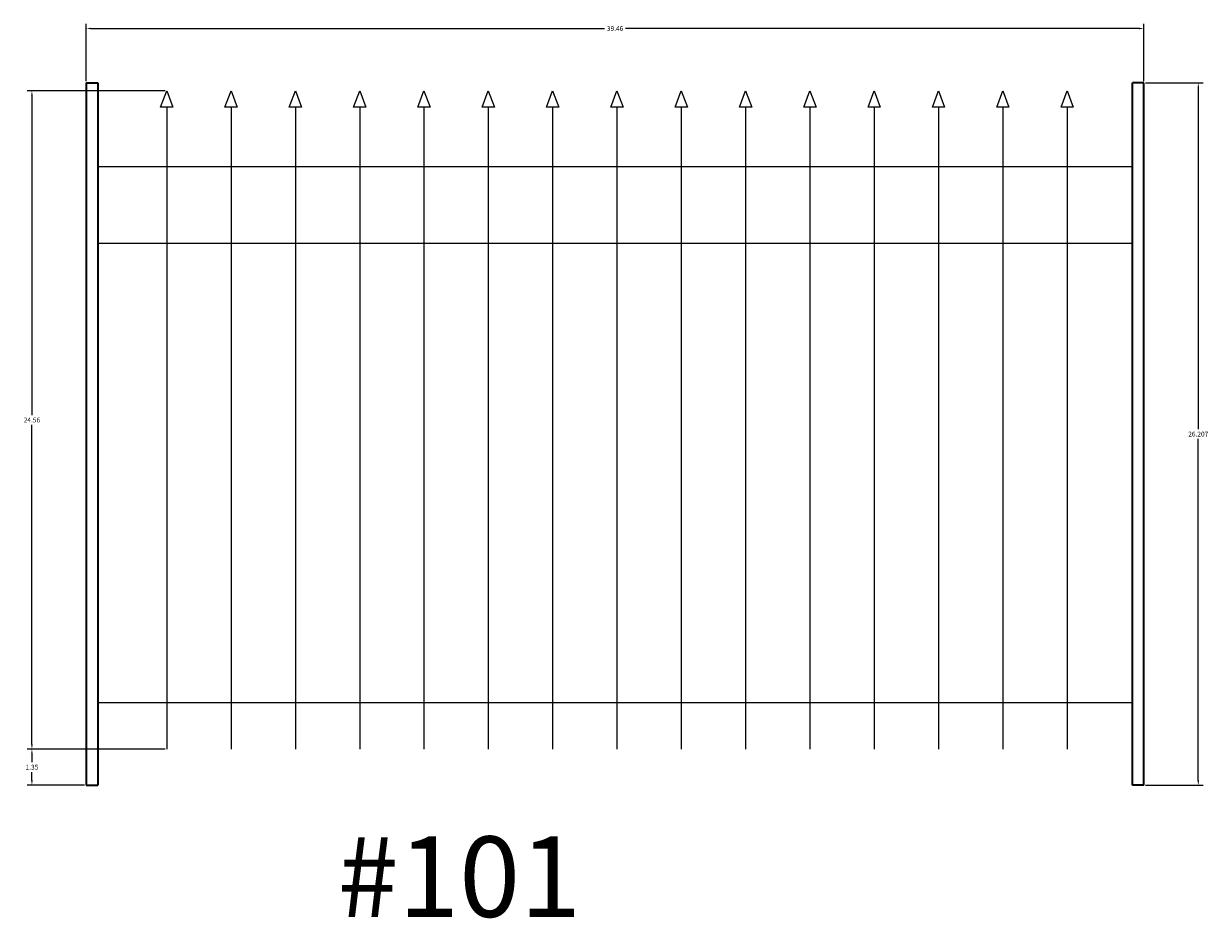
# Model space of a CAD drawing. Units: inches. Extents: x 756 to 915, y 488 to 695.
# Tile 20 of 25: x 815 to 859, y 661 to 694. Entities that reach past the tile are written whole.
import ezdxf

# ---------------------------------------------------------------- set-up
doc = ezdxf.new("R2010")
doc.units = ezdxf.units.IN
doc.header["$MEASUREMENT"] = 0
for name, color, linetype, lineweight in [('L-ANNO-TEXT', 7, 'Continuous', 25), ('L-FENC-PCKT', 7, 'Continuous', 18), ('L-FENC-POST', 7, 'Continuous', 35), ('L-FENC-RAIL', 7, 'Continuous', 25), ('M-DIMS', 2, 'Continuous', 18)]:
    doc.layers.add(name, color=color, linetype=linetype, lineweight=lineweight)
doc.styles.get("Standard").update_dxf_attribs({"font": 'arial.ttf'})
doc.dimstyles.get("Standard").update_dxf_attribs({"dimtxt": 0.18, "dimasz": 0.18, "dimexe": 0.18, "dimexo": 0.0625, "dimgap": 0.09, "dimtad": 0, "dimtih": 1, "dimtoh": 1, "dimdec": 0, "dimzin": 0, "dimdsep": 46, "dimlunit": 3, "dimtxsty": 'Standard', "dimcen": 0.09, "dimadec": 0, "dimazin": 0, "dimtfac": 1, "dimtdec": 0, "dimtofl": 0, "dimtmove": 0, "dimatfit": 3, "dimfxl": 1, "dimtolj": 1, "dimtzin": 0, "dimarcsym": 0})

# ---------------------------------------------------------------- blocks, each defined once
blk = doc.blocks.new('PICKET-SPEAR-EXTENDED')
blk.add_line((0.228, 23.946), (0.228, 0))
blk.add_lwpolyline([(0.228, 23.946), (0, 23.946), (0.228, 24.558), (0.455, 23.946)], close=True)
blk = doc.blocks.new('FENCE-POST-LEFT')
for p, q in [((0, 26.207), (0, 0)), ((0, 26.207), (0.426, 26.207)), ((0.426, 26.207), (0.426, 0)), ((0.426, 26.207), (0.426, 0)), ((0, 0), (0.426, 0))]:
    blk.add_line(p, q)
blk = doc.blocks.new('FENCE-POST-RIGHT')
for p, q in [((0, 26.207), (0, 0)), ((0, 26.207), (0.427, 26.207)), ((0.427, 26.207), (0.427, 0)), ((0, 0), (0.427, 0))]:
    blk.add_line(p, q)
blk = doc.blocks.new('*D19')
at = {"layer": 'Defpoints', "color": 0, "transparency": 16777216}
for p in [(856.698, 693.983), (817.24, 691.953), (856.698, 691.953)]:
    blk.add_point(p, dxfattribs=at)
at = {"layer": 'M-DIMS', "color": 0, "lineweight": -2, "transparency": 16777216}
for p, q in [((817.24, 692.015), (817.24, 694.163)), ((817.42, 693.983), (836.575, 693.983)), ((856.518, 693.983), (837.362, 693.983)), ((856.698, 692.015), (856.698, 694.163))]:
    blk.add_line(p, q, dxfattribs=at)
at = {"layer": 'M-DIMS', "color": 0, "transparency": 16777216}
for points in [[(817.42, 694.013), (817.42, 693.953), (817.24, 693.983)], [(856.518, 694.013), (856.518, 693.953), (856.698, 693.983)]]:
    blk.add_solid(points, dxfattribs=at)
at = {"layer": 'M-DIMS', "color": 0, "transparency": 16777216, "insert": (836.969, 693.983), "char_height": 0.18, "attachment_point": 5}
blk.add_mtext('\\A1;39.46', dxfattribs=at)
blk = doc.blocks.new('*D20')
at = {"layer": 'Defpoints', "color": 0, "transparency": 16777216}
for p in [(856.698, 691.953), (858.728, 691.953), (856.698, 665.746)]:
    blk.add_point(p, dxfattribs=at)
at = {"layer": 'M-DIMS', "color": 0, "lineweight": -2, "transparency": 16777216}
for p, q in [((856.76, 691.953), (858.908, 691.953)), ((858.728, 691.773), (858.728, 679.031)), ((858.728, 665.926), (858.728, 678.668)), ((856.76, 665.746), (858.908, 665.746))]:
    blk.add_line(p, q, dxfattribs=at)
at = {"layer": 'M-DIMS', "color": 0, "transparency": 16777216}
for points in [[(858.698, 691.773), (858.758, 691.773), (858.728, 691.953)], [(858.698, 665.926), (858.758, 665.926), (858.728, 665.746)]]:
    blk.add_solid(points, dxfattribs=at)
at = {"layer": 'M-DIMS', "color": 0, "transparency": 16777216, "insert": (858.728, 678.849), "char_height": 0.18, "attachment_point": 5}
blk.add_mtext('\\A1;26.207', dxfattribs=at)
blk = doc.blocks.new('*D21')
at = {"layer": 'Defpoints', "color": 0, "transparency": 16777216}
for p in [(815.21, 691.654), (820.239, 691.654), (820.239, 667.096)]:
    blk.add_point(p, dxfattribs=at)
at = {"layer": 'M-DIMS', "color": 0, "lineweight": -2, "transparency": 16777216}
for p, q in [((820.176, 691.654), (815.03, 691.654)), ((815.21, 691.474), (815.21, 679.557)), ((815.21, 667.276), (815.21, 679.193)), ((820.176, 667.096), (815.03, 667.096))]:
    blk.add_line(p, q, dxfattribs=at)
at = {"layer": 'M-DIMS', "color": 0, "transparency": 16777216}
for points in [[(815.18, 691.474), (815.24, 691.474), (815.21, 691.654)], [(815.18, 667.276), (815.24, 667.276), (815.21, 667.096)]]:
    blk.add_solid(points, dxfattribs=at)
at = {"layer": 'M-DIMS', "color": 0, "transparency": 16777216, "insert": (815.21, 679.375), "char_height": 0.18, "attachment_point": 5}
blk.add_mtext('\\A1;24.56', dxfattribs=at)
blk = doc.blocks.new('*D22')
at = {"layer": 'Defpoints', "color": 0, "transparency": 16777216}
for p in [(815.21, 667.096), (820.239, 667.096), (817.24, 665.746)]:
    blk.add_point(p, dxfattribs=at)
at = {"layer": 'M-DIMS', "color": 0, "lineweight": -2, "transparency": 16777216}
for p, q in [((820.176, 667.096), (815.03, 667.096)), ((815.21, 666.916), (815.21, 666.603)), ((815.21, 665.926), (815.21, 666.239)), ((817.177, 665.746), (815.03, 665.746))]:
    blk.add_line(p, q, dxfattribs=at)
at = {"layer": 'M-DIMS', "color": 0, "transparency": 16777216}
for points in [[(815.18, 666.916), (815.24, 666.916), (815.21, 667.096)], [(815.18, 665.926), (815.24, 665.926), (815.21, 665.746)]]:
    blk.add_solid(points, dxfattribs=at)
at = {"layer": 'M-DIMS', "color": 0, "transparency": 16777216, "insert": (815.21, 666.421), "char_height": 0.18, "attachment_point": 5}
blk.add_mtext('\\A1;1.35', dxfattribs=at)

msp = doc.modelspace()

# ---------------------------------------------------------------- linework, layer by layer
at = {"layer": 'L-FENC-RAIL'}
for p, q in [((817.6662, 688.8379), (856.271, 688.8379)), ((817.6662, 685.9735), (856.271, 685.9735)), ((817.6662, 668.8277), (856.271, 668.8277))]:
    msp.add_line(p, q, dxfattribs=at)

# ---------------------------------------------------------------- block references
at = {"layer": 'L-FENC-PCKT'}
for p in [(820.011, 667.096), (822.4109, 667.096), (824.8108, 667.096), (827.2108, 667.096), (829.6107, 667.096), (832.0106, 667.096), (834.4105, 667.096), (836.8104, 667.096), (839.2103, 667.096), (841.6102, 667.096), (844.0101, 667.096), (846.41, 667.096), (848.81, 667.096), (851.2099, 667.096), (853.6098, 667.096)]:
    msp.add_blockref('PICKET-SPEAR-EXTENDED', p, dxfattribs=at)
at = {"layer": 'L-FENC-POST'}
msp.add_blockref('FENCE-POST-LEFT', (817.2399, 665.746), dxfattribs=at)
at = {"layer": 'L-FENC-POST', "rotation": 180}
msp.add_blockref('FENCE-POST-RIGHT', (856.6978, 691.9529), dxfattribs=at)

# ---------------------------------------------------------------- texts
at = {"layer": 'L-ANNO-TEXT'}
msp.add_text('#101', height=3, dxfattribs=at).set_placement((826.6109, 660.8341))

# ---------------------------------------------------------------- dimensions: what is measured, and where the dimension line sits
at = {"layer": 'M-DIMS'}
dim = msp.add_linear_dim(base=(856.6977, 693.9829), p1=(817.2395, 691.9529), p2=(856.6977, 691.9529), dimstyle='Standard', override={"dimdec": 2, "dimlfac": 1, "dimrnd": 0, "dimzin": 0, "dimdsep": 46, "dimlunit": 2}, dxfattribs=at)
dim.commit()
dim.dimension.update_dxf_attribs({"geometry": '*D19', "text_midpoint": (836.9686, 693.9829)})
for base, p1, p2, override, picture, middle in [((858.7277, 691.9529), (856.6977, 665.7461), (856.6977, 691.9529), {"dimdec": 3, "dimlfac": 1, "dimrnd": 0, "dimzin": 0, "dimdsep": 46, "dimlunit": 2}, '*D20', (858.7277, 678.8495)), ((815.2095, 691.6538), (820.2387, 667.0956), (820.2387, 691.6538), {"dimdec": 2, "dimlfac": 1, "dimrnd": 0, "dimzin": 0, "dimdsep": 46, "dimlunit": 2}, '*D21', (815.2095, 679.3747)), ((815.2095, 667.0956), (817.2395, 665.7461), (820.2387, 667.0956), {"dimdec": 2, "dimlfac": 1, "dimrnd": 0, "dimzin": 0, "dimdsep": 46, "dimlunit": 2}, '*D22', (815.2095, 666.4208))]:
    dim = msp.add_linear_dim(base=base, p1=p1, p2=p2, angle=90, dimstyle='Standard', override=override, dxfattribs=at)
    dim.commit()
    dim.dimension.update_dxf_attribs({"geometry": picture, "text_midpoint": middle})

doc.saveas('drawing.dxf')
